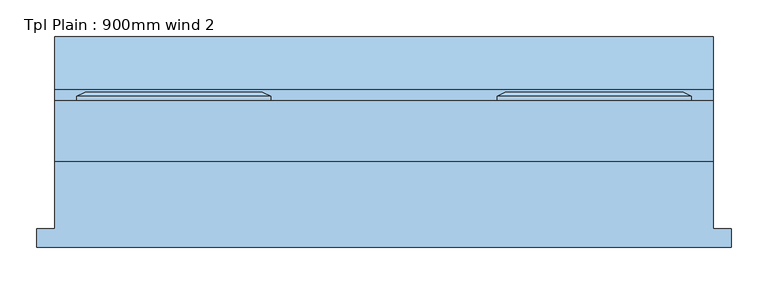
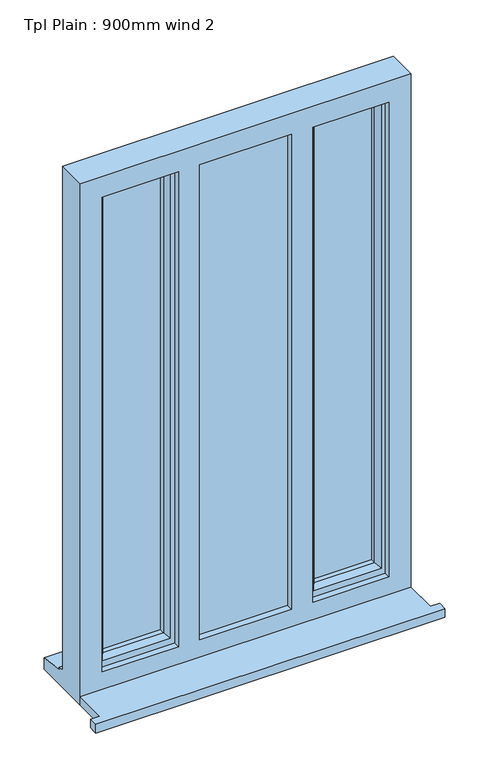
"""IFC4 building model written with IfcOpenShell, lengths in millimetres: window geometry, Tpl Plain : 900mm wind 2."""

from ifc_helpers import new_model, si_unit, frame, origin, place, context, project, spatial, polyline, outline, extrude, faceted_brep, source, transform, mapped, element, save


def tpl_plain_900mm_wind_2_fce8a64c(model_context):
    return source(origin(), model_context, "Body", "SolidModel", [
        extrude(outline(polyline([(-900.0, -129.0434322), (-900.0, -104.0434322), (-875.0, -104.0434322), (-875.0, -12.0434322), (25.0, -12.0434322), (25.0, -104.0434322), (50.0, -104.0434322), (50.0, -129.0434322), (-900.0, -129.0434322)])), frame((0.0, 0.0, 900.0), z_axis=(0.0, 0.0, 1.0), x_axis=(1.0, 0.0, 0.0)), (0.0, 0.0, 1.0), 25.0),
        faceted_brep([(-270.0, 70.9565678, 2370.0), (-270.0, 76.7300705, 2370.0), (-270.0, 76.7300705, 953.0), (-270.0, 70.9565678, 953.0), (-260.0, 5.9565678, 2360.0), (-260.0, 70.9565678, 2360.0), (-260.0, 70.9565678, 963.0), (-260.0, 5.9565678, 963.0), (-220.0, 20.4494677, 2320.0), (-230.1480377, 5.9565678, 2330.1480377), (-230.1480377, 5.9565678, 992.8519623), (-220.0, 20.4494677, 1003.0), (-220.0, 34.9565678, 2320.0), (-220.0, 34.9565678, 1003.0), (-230.0, 58.9565678, 2330.0), (-230.0, 34.9565678, 2330.0), (-230.0, 34.9565678, 993.0), (-230.0, 58.9565678, 993.0), (-220.0, 76.7300705, 2320.0), (-220.0, 58.9565678, 2320.0), (-220.0, 58.9565678, 1003.0), (-220.0, 76.7300705, 1003.0), (-237.4457548, 82.5035732, 2337.4457548), (-237.4457548, 82.5035732, 985.5542452), (-259.2153903, 82.5035732, 2359.2153903), (-259.2153903, 82.5035732, 963.7846097), (-5.0, 76.7300705, 953.0), (-5.0, 70.9565678, 953.0), (-15.0, 70.9565678, 963.0), (-15.0, 5.9565678, 963.0), (-44.8519623, 5.9565678, 992.8519623), (-55.0, 20.4494677, 1003.0), (-55.0, 34.9565678, 1003.0), (-45.0, 34.9565678, 993.0), (-45.0, 58.9565678, 993.0), (-55.0, 58.9565678, 1003.0), (-55.0, 76.7300705, 1003.0), (-37.5542452, 82.5035732, 985.5542452), (-15.7846097, 82.5035732, 963.7846097), (-5.0, 76.7300705, 2370.0), (-5.0, 70.9565678, 2370.0), (-15.0, 70.9565678, 2360.0), (-15.0, 5.9565678, 2360.0), (-44.8519623, 5.9565678, 2330.1480377), (-55.0, 20.4494677, 2320.0), (-55.0, 34.9565678, 2320.0), (-45.0, 34.9565678, 2330.0), (-45.0, 58.9565678, 2330.0), (-55.0, 58.9565678, 2320.0), (-55.0, 76.7300705, 2320.0), (-37.5542452, 82.5035732, 2337.4457548), (-15.7846097, 82.5035732, 2359.2153903)], [[[0, 1, 2, 3]], [[4, 5, 6, 7]], [[8, 9, 10, 11]], [[12, 8, 11, 13]], [[14, 15, 16, 17]], [[18, 19, 20, 21]], [[22, 18, 21, 23]], [[1, 24, 25, 2]], [[3, 2, 26, 27]], [[7, 6, 28, 29]], [[11, 10, 30, 31]], [[13, 11, 31, 32]], [[17, 16, 33, 34]], [[21, 20, 35, 36]], [[23, 21, 36, 37]], [[2, 25, 38, 26]], [[27, 26, 39, 40]], [[29, 28, 41, 42]], [[31, 30, 43, 44]], [[32, 31, 44, 45]], [[34, 33, 46, 47]], [[36, 35, 48, 49]], [[37, 36, 49, 50]], [[26, 38, 51, 39]], [[40, 39, 1, 0]], [[3, 27, 40, 0], [5, 41, 28, 6]], [[42, 41, 5, 4]], [[7, 29, 42, 4], [9, 43, 30, 10]], [[44, 43, 9, 8]], [[45, 44, 8, 12]], [[15, 46, 33, 16], [13, 32, 45, 12]], [[47, 46, 15, 14]], [[17, 34, 47, 14], [19, 48, 35, 20]], [[49, 48, 19, 18]], [[50, 49, 18, 22]], [[24, 51, 38, 25], [23, 37, 50, 22]], [[39, 51, 24, 1]]]),
        faceted_brep([(-580.0, 70.9565678, 2370.0), (-580.0, 76.7300705, 2370.0), (-845.0, 76.7300705, 2370.0), (-845.0, 70.9565678, 2370.0), (-590.0, 5.9565678, 2360.0), (-590.0, 70.9565678, 2360.0), (-835.0, 70.9565678, 2360.0), (-835.0, 5.9565678, 2360.0), (-630.0, 20.4494677, 2320.0), (-619.8519623, 5.9565678, 2330.1480377), (-805.1480377, 5.9565678, 2330.1480377), (-795.0, 20.4494677, 2320.0), (-630.0, 34.9565678, 2320.0), (-795.0, 34.9565678, 2320.0), (-620.0, 58.9565678, 2330.0), (-620.0, 34.9565678, 2330.0), (-805.0, 34.9565678, 2330.0), (-805.0, 58.9565678, 2330.0), (-630.0, 76.7300705, 2320.0), (-630.0, 58.9565678, 2320.0), (-795.0, 58.9565678, 2320.0), (-795.0, 76.7300705, 2320.0), (-611.1854344, 82.5035732, 2338.8145656), (-813.8145656, 82.5035732, 2338.8145656), (-591.6307806, 82.5035732, 2358.3692194), (-833.3692194, 82.5035732, 2358.3692194), (-845.0, 76.7300705, 953.0), (-845.0, 70.9565678, 953.0), (-835.0, 70.9565678, 963.0), (-835.0, 5.9565678, 963.0), (-805.1480377, 5.9565678, 992.8519623), (-795.0, 20.4494677, 1003.0), (-795.0, 34.9565678, 1003.0), (-805.0, 34.9565678, 993.0), (-805.0, 58.9565678, 993.0), (-795.0, 58.9565678, 1003.0), (-795.0, 76.7300705, 1003.0), (-813.8145656, 82.5035732, 984.1854344), (-833.3692194, 82.5035732, 964.6307806), (-580.0, 76.7300705, 953.0), (-580.0, 70.9565678, 953.0), (-590.0, 70.9565678, 963.0), (-590.0, 5.9565678, 963.0), (-619.8519623, 5.9565678, 992.8519623), (-630.0, 20.4494677, 1003.0), (-630.0, 34.9565678, 1003.0), (-620.0, 34.9565678, 993.0), (-620.0, 58.9565678, 993.0), (-630.0, 58.9565678, 1003.0), (-630.0, 76.7300705, 1003.0), (-611.1854344, 82.5035732, 984.1854344), (-591.6307806, 82.5035732, 964.6307806)], [[[0, 1, 2, 3]], [[4, 5, 6, 7]], [[8, 9, 10, 11]], [[12, 8, 11, 13]], [[14, 15, 16, 17]], [[18, 19, 20, 21]], [[22, 18, 21, 23]], [[1, 24, 25, 2]], [[3, 2, 26, 27]], [[7, 6, 28, 29]], [[11, 10, 30, 31]], [[13, 11, 31, 32]], [[17, 16, 33, 34]], [[21, 20, 35, 36]], [[23, 21, 36, 37]], [[2, 25, 38, 26]], [[27, 26, 39, 40]], [[0, 3, 27, 40], [41, 28, 6, 5]], [[29, 28, 41, 42]], [[4, 7, 29, 42], [43, 30, 10, 9]], [[31, 30, 43, 44]], [[32, 31, 44, 45]], [[46, 33, 16, 15], [12, 13, 32, 45]], [[34, 33, 46, 47]], [[14, 17, 34, 47], [48, 35, 20, 19]], [[36, 35, 48, 49]], [[37, 36, 49, 50]], [[51, 38, 25, 24], [22, 23, 37, 50]], [[26, 38, 51, 39]], [[40, 39, 1, 0]], [[42, 41, 5, 4]], [[44, 43, 9, 8]], [[45, 44, 8, 12]], [[47, 46, 15, 14]], [[49, 48, 19, 18]], [[50, 49, 18, 22]], [[39, 51, 24, 1]]]),
        faceted_brep([(25.0, -12.0434322, 2400.0), (-875.0, -12.0434322, 2400.0), (-875.0, -12.0434322, 900.0), (25.0, -12.0434322, 900.0), (-35.0, -12.0434322, 2340.0), (-35.0, -12.0434322, 975.0), (-242.0, -12.0434322, 975.0), (-242.0, -12.0434322, 2340.0), (-300.0, -12.0434322, 2340.0), (-300.0, -12.0434322, 975.0), (-550.0, -12.0434322, 975.0), (-550.0, -12.0434322, 2340.0), (-608.0, -12.0434322, 2340.0), (-608.0, -12.0434322, 975.0), (-815.0, -12.0434322, 975.0), (-815.0, -12.0434322, 2340.0), (-875.0, 70.9565678, 2400.0), (-875.0, 70.9565678, 951.0), (-875.0, 85.9565678, 949.68767), (-875.0, 85.9565678, 944.7449676), (-875.0, 158.4565678, 933.8088847), (-875.0, 158.4565678, 900.0), (25.0, 70.9565678, 2400.0), (25.0, 70.9565678, 951.0), (-835.0, 70.9565678, 2360.0), (-835.0, 70.9565678, 963.0), (-590.0, 70.9565678, 963.0), (-590.0, 70.9565678, 2360.0), (-550.0, 70.9565678, 2360.0), (-550.0, 70.9565678, 963.0), (-300.0, 70.9565678, 963.0), (-300.0, 70.9565678, 2360.0), (-260.0, 70.9565678, 2360.0), (-260.0, 70.9565678, 963.0), (-15.0, 70.9565678, 963.0), (-15.0, 70.9565678, 2360.0), (-835.0, 5.9565678, 2360.0), (-835.0, 5.9565678, 963.0), (-560.0, 5.9565678, 2360.0), (-290.0, 5.9565678, 2360.0), (-290.0, 5.9565678, 963.0), (-560.0, 5.9565678, 963.0), (-300.0, 5.9565678, 2340.0), (-550.0, 5.9565678, 2340.0), (-550.0, 5.9565678, 975.0), (-300.0, 5.9565678, 975.0), (-260.0, 5.9565678, 2360.0), (-15.0, 5.9565678, 2360.0), (-15.0, 5.9565678, 963.0), (-260.0, 5.9565678, 963.0), (-35.0, 5.9565678, 2340.0), (-242.0, 5.9565678, 2340.0), (-242.0, 5.9565678, 975.0), (-35.0, 5.9565678, 975.0), (-590.0, 5.9565678, 2360.0), (-590.0, 5.9565678, 963.0), (-608.0, 5.9565678, 2340.0), (-815.0, 5.9565678, 2340.0), (-815.0, 5.9565678, 975.0), (-608.0, 5.9565678, 975.0), (-550.0, 29.9565678, 2360.0), (-300.0, 29.9565678, 2360.0), (-290.0, 29.9565678, 2360.0), (-560.0, 29.9565678, 2360.0), (25.0, 158.4565678, 900.0), (25.0, 158.4565678, 933.8088847), (25.0, 85.9565678, 944.7449676), (25.0, 85.9565678, 949.68767), (-550.0, 29.9565678, 963.0), (-560.0, 29.9565678, 963.0), (-290.0, 29.9565678, 963.0), (-300.0, 29.9565678, 963.0)], [[[0, 1, 2, 3], [4, 5, 6, 7], [8, 9, 10, 11], [12, 13, 14, 15]], [[2, 1, 16, 17, 18, 19, 20, 21]], [[17, 16, 22, 23], [24, 25, 26, 27], [28, 29, 30, 31], [32, 33, 34, 35]], [[25, 24, 36, 37]], [[38, 39, 40, 41], [42, 43, 44, 45]], [[46, 47, 48, 49], [50, 51, 52, 53]], [[36, 54, 55, 37], [56, 57, 58, 59]], [[57, 15, 14, 58]], [[1, 0, 22, 16]], [[36, 24, 27, 54]], [[35, 47, 46, 32]], [[60, 28, 31, 61, 62, 39, 38, 63]], [[15, 57, 56, 12]], [[50, 4, 7, 51]], [[11, 43, 42, 8]], [[23, 22, 0, 3, 64, 65, 66, 67]], [[35, 34, 48, 47]], [[4, 50, 53, 5]], [[43, 11, 10, 44]], [[12, 56, 59, 13]], [[27, 26, 55, 54]], [[29, 28, 60, 68]], [[68, 60, 63, 69]], [[69, 63, 38, 41]], [[62, 70, 40, 39]], [[70, 62, 61, 71]], [[71, 61, 31, 30]], [[33, 32, 46, 49]], [[51, 7, 6, 52]], [[8, 42, 45, 9]], [[64, 3, 2, 21]], [[65, 64, 21, 20]], [[66, 65, 20, 19]], [[67, 66, 19, 18]], [[23, 67, 18, 17]], [[26, 25, 37, 55]], [[34, 33, 49, 48]], [[41, 40, 70, 71, 30, 29, 68, 69]], [[6, 5, 53, 52]], [[45, 44, 10, 9]], [[59, 58, 14, 13]]]),
        extrude(outline(polyline([(-620.0, 34.9565678), (-805.0, 34.9565678), (-805.0, 58.9565678), (-620.0, 58.9565678), (-620.0, 34.9565678)])), frame((0.0, 0.0, 993.0), z_axis=(0.0, 0.0, 1.0), x_axis=(1.0, 0.0, 0.0)), (0.0, 0.0, 1.0), 1337.0),
        extrude(outline(polyline([(-560.0, 29.9565678), (-290.0, 29.9565678), (-290.0, 5.9565678), (-560.0, 5.9565678), (-560.0, 29.9565678)])), frame((0.0, 0.0, 963.0), z_axis=(0.0, 0.0, 1.0), x_axis=(1.0, 0.0, 0.0)), (0.0, 0.0, 1.0), 1397.0),
        extrude(outline(polyline([(-45.0, 34.9565678), (-230.0, 34.9565678), (-230.0, 58.9565678), (-45.0, 58.9565678), (-45.0, 34.9565678)])), frame((0.0, 0.0, 993.0), z_axis=(0.0, 0.0, 1.0), x_axis=(1.0, 0.0, 0.0)), (0.0, 0.0, 1.0), 1337.0),
    ])


if __name__ == "__main__":
    model = new_model("IFC4")
    model_context = context("Model", 3, world=origin())
    ifc_project = project(units=[si_unit("LENGTHUNIT", "METRE", prefix="MILLI")], contexts=[model_context])
    site = spatial("IfcSite", under=ifc_project)
    building = spatial("IfcBuilding", under=site)
    placement = place(None, origin())
    tpl_plain_900mm_wind_2_shape = tpl_plain_900mm_wind_2_fce8a64c(model_context)
    element("IfcWindow", 1, ObjectType="Tpl Plain : 900mm wind 2", at=placement, inside=building, context=model_context, shape_type="MappedRepresentation", body=[
        mapped(tpl_plain_900mm_wind_2_shape, transform((0.0, 0.0, 0.0), x_axis=(1.0, 0.0, 0.0), y_axis=(0.0, 1.0, 0.0), z_axis=(0.0, 0.0, 1.0))),
    ])
    save(model, "model.ifc")

# Revit data of these elements
# Type "Tpl Plain : 900mm wind 2"
#   Type Mark = "36"
#   Operation = "TriplePanelVertical"
#   Manufacturer = "Revit"
#   Keynote = "L10"
#   Analytic Construction = "<None>"
#   Wrap Layers (Ext) from Ext = 102.5 mm
#   Wrap Layers (Int) from Ext = 177.5 mm
#   Window Board Projection = 25 mm
#   Window Board Extension = 25 mm
#   Rough Width = 900 mm
#   Rough Height = 1500 mm
#   Height = 1500 mm
#   Width = 900 mm
#   Glazing Thickness = 24 mm
#   FrameOffset - External = 50 mm
#   Frame Depth = 65 mm
#   Default Head Height = 2400 mm
#   Cill Depth = 87.5 mm
#   Cavity Closer Width = 50 mm
#   Cavity Closer Offset from Ext = 102.5 mm
#   Cavity Closer Depth = 85 mm
#   Vis - Cavity Closers = yes
#   Define Thermal Properties by = 1
#   Material Trim = Window Frame
#   Material Glass = Glass
#   Material Frame = Window Frame
#   Wall Closure = (empty or 0)
# Element 1 (IfcWindow, "Tpl Plain : 900mm wind 2")
#   Materials on its faces: "Window Frame", "Glass"
# Materials
#   "Window Frame": colour RGB 249 249 249, transparency 0, Keynote = "L10", Cost = 0
#   "Glass": class "Glass", colour RGB 0 128 192, transparency 0.9, Description = "Soda Lime Glass", Cost = 0
